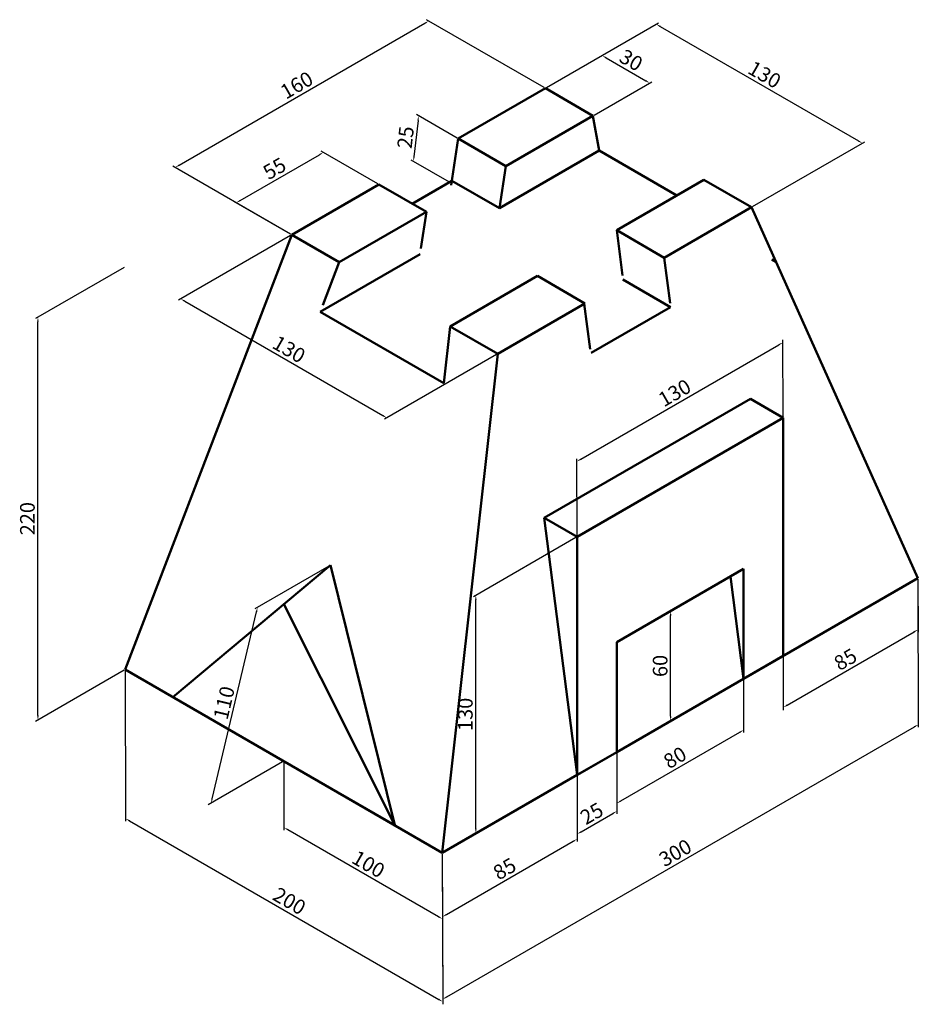
# Model space of a CAD drawing. Units: millimetres. Extents: x 46 to 537, y -102 to 436.
import ezdxf

# ---------------------------------------------------------------- set-up
doc = ezdxf.new("R2010")
doc.units = ezdxf.units.MM
doc.layers.add('M-DIMS', color=3, linetype='Continuous', lineweight=25)
doc.layers.add('M-OUTL', color=7, linetype='Continuous', lineweight=50)
doc.styles.get("Standard").update_dxf_attribs({"font": 'arial.ttf'})
doc.dimstyles.new('ISO-25', dxfattribs={"dimtxt": 8, "dimasz": 2.5, "dimexe": 1.25, "dimexo": 0.625, "dimtad": 1, "dimtxsty": 'Standard', "dimcen": 2.5, "dimadec": 0, "dimazin": 0, "dimtfac": 1, "dimtmove": 0, "dimatfit": 3, "dimfxl": 1, "dimarcsym": 0})

# ---------------------------------------------------------------- blocks, each defined once
blk = doc.blocks.new('*D1')
at = {"layer": 'Defpoints', "color": 0, "transparency": 16777216}
for p in [(333.35, 398.34), (390.34, 401.24), (359.33, 383.34)]:
    blk.add_point(p, dxfattribs=at)
at = {"layer": 'M-DIMS', "color": 0, "lineweight": -2, "transparency": 16777216}
for p, q in [((333.98, 398.7), (365.61, 416.96)), ((366.52, 414.99), (388.17, 402.49)), ((359.96, 383.7), (391.59, 401.96))]:
    blk.add_line(p, q, dxfattribs=at)
at = {"layer": 'M-DIMS', "color": 0, "transparency": 16777216}
for points in [[(366.73, 415.35), (366.32, 414.63), (364.36, 416.24)], [(388.38, 402.85), (387.97, 402.13), (390.34, 401.24)]]:
    blk.add_solid(points, dxfattribs=at)
at = {"layer": 'M-DIMS', "color": 0, "transparency": 16777216, "insert": (379.71, 412.82), "char_height": 8, "attachment_point": 5, "rotation": 330}
blk.add_mtext('30', dxfattribs=at)
blk = doc.blocks.new('*D2')
at = {"layer": 'Defpoints', "color": 0, "transparency": 16777216}
for p in [(333.35, 398.34), (506.56, 368.34), (445.93, 333.34)]:
    blk.add_point(p, dxfattribs=at)
at = {"layer": 'M-DIMS', "color": 0, "lineweight": -2, "transparency": 16777216}
for p, q in [((333.98, 398.7), (395.22, 434.06)), ((396.14, 432.09), (504.39, 369.59)), ((446.56, 333.7), (507.81, 369.06))]:
    blk.add_line(p, q, dxfattribs=at)
at = {"layer": 'M-DIMS', "color": 0, "transparency": 16777216}
for points in [[(396.35, 432.45), (395.93, 431.72), (393.97, 433.34)], [(504.6, 369.95), (504.18, 369.22), (506.56, 368.34)]]:
    blk.add_solid(points, dxfattribs=at)
at = {"layer": 'M-DIMS', "color": 0, "transparency": 16777216, "insert": (452.62, 404.92), "char_height": 8, "attachment_point": 5, "rotation": 330}
blk.add_mtext('130', dxfattribs=at)
blk = doc.blocks.new('*D3')
at = {"layer": 'Defpoints', "color": 0, "transparency": 16777216}
for p in [(212.11, 363.34), (242.42, 345.84), (194.79, 318.34)]:
    blk.add_point(p, dxfattribs=at)
at = {"layer": 'M-DIMS', "color": 0, "lineweight": -2, "transparency": 16777216}
for p, q in [((166.64, 337.09), (209.94, 362.09)), ((241.79, 346.2), (210.86, 364.06)), ((194.16, 318.7), (163.23, 336.56))]:
    blk.add_line(p, q, dxfattribs=at)
at = {"layer": 'M-DIMS', "color": 0, "transparency": 16777216}
for points in [[(209.73, 362.45), (210.15, 361.72), (212.11, 363.34)], [(166.43, 337.45), (166.85, 336.72), (164.48, 335.84)]]:
    blk.add_solid(points, dxfattribs=at)
at = {"layer": 'M-DIMS', "color": 0, "transparency": 16777216, "insert": (185.94, 353.65), "char_height": 8, "attachment_point": 5, "rotation": 30}
blk.add_mtext('55', dxfattribs=at)
blk = doc.blocks.new('*D4')
at = {"layer": 'Defpoints', "color": 0, "transparency": 16777216}
for p in [(285.72, 370.84), (261.3, 358.47), (282.91, 345.99)]:
    blk.add_point(p, dxfattribs=at)
at = {"layer": 'M-DIMS', "color": 0, "lineweight": -2, "transparency": 16777216}
for p, q in [((285.13, 371.18), (262.92, 384)), ((263.82, 380.83), (261.58, 360.96)), ((282.32, 346.33), (260.12, 359.15))]:
    blk.add_line(p, q, dxfattribs=at)
at = {"layer": 'M-DIMS', "color": 0, "transparency": 16777216}
for points in [[(263.41, 380.88), (264.24, 380.78), (264.1, 383.31)], [(261.17, 361), (261.99, 360.91), (261.3, 358.47)]]:
    blk.add_solid(points, dxfattribs=at)
at = {"layer": 'M-DIMS', "color": 0, "transparency": 16777216, "insert": (258.02, 371.42), "char_height": 8, "attachment_point": 5, "rotation": 83.5591}
blk.add_mtext('25', dxfattribs=at)
blk = doc.blocks.new('*D5')
at = {"layer": 'Defpoints', "color": 0, "transparency": 16777216}
for p in [(103.85, 300.84), (56.16, 273.3), (103.85, 80.84)]:
    blk.add_point(p, dxfattribs=at)
at = {"layer": 'M-DIMS', "color": 0, "lineweight": -2, "transparency": 16777216}
for p, q in [((103.23, 300.47), (54.91, 272.58)), ((56.16, 55.8), (56.16, 270.8)), ((103.23, 80.47), (54.91, 52.58))]:
    blk.add_line(p, q, dxfattribs=at)
at = {"layer": 'M-DIMS', "color": 0, "transparency": 16777216}
for points in [[(55.74, 270.8), (56.57, 270.8), (56.16, 273.3)], [(55.74, 55.8), (56.57, 55.8), (56.16, 53.3)]]:
    blk.add_solid(points, dxfattribs=at)
at = {"layer": 'M-DIMS', "color": 0, "transparency": 16777216, "insert": (51.45, 163.3), "char_height": 8, "attachment_point": 5, "rotation": 90}
blk.add_mtext('220', dxfattribs=at)
blk = doc.blocks.new('*D6')
at = {"layer": 'Defpoints', "color": 0, "transparency": 16777216}
for p in [(103.85, 80.84), (277.06, -19.16), (277.29, -100.49)]:
    blk.add_point(p, dxfattribs=at)
at = {"layer": 'M-DIMS', "color": 0, "lineweight": -2, "transparency": 16777216}
for p, q in [((103.86, 80.11), (104.09, -1.93)), ((106.25, -1.74), (275.13, -99.24)), ((277.06, -19.89), (277.3, -101.93))]:
    blk.add_line(p, q, dxfattribs=at)
at = {"layer": 'M-DIMS', "color": 0, "transparency": 16777216}
for points in [[(106.46, -1.38), (106.04, -2.1), (104.09, -0.49)], [(275.33, -98.88), (274.92, -99.6), (277.29, -100.49)]]:
    blk.add_solid(points, dxfattribs=at)
at = {"layer": 'M-DIMS', "color": 0, "transparency": 16777216, "insert": (193.04, -46.41), "char_height": 8, "attachment_point": 5, "rotation": 330}
blk.add_mtext('200', dxfattribs=at)
blk = doc.blocks.new('*D7')
at = {"layer": 'Defpoints', "color": 0, "transparency": 16777216}
for p in [(190.46, 30.84), (190.56, -5.35), (277.06, -19.16)]:
    blk.add_point(p, dxfattribs=at)
at = {"layer": 'M-DIMS', "color": 0, "lineweight": -2, "transparency": 16777216}
for p, q in [((190.46, 30.11), (190.56, -6.8)), ((275, -54.1), (192.72, -6.6)), ((277.06, -19.89), (277.17, -56.8))]:
    blk.add_line(p, q, dxfattribs=at)
at = {"layer": 'M-DIMS', "color": 0, "transparency": 16777216}
for points in [[(192.93, -6.24), (192.52, -6.96), (190.56, -5.35)], [(275.21, -53.74), (274.79, -54.46), (277.16, -55.35)]]:
    blk.add_solid(points, dxfattribs=at)
at = {"layer": 'M-DIMS', "color": 0, "transparency": 16777216, "insert": (236.22, -26.27), "char_height": 8, "attachment_point": 5, "rotation": 330}
blk.add_mtext('100', dxfattribs=at)
blk = doc.blocks.new('*D8')
at = {"layer": 'Defpoints', "color": 0, "transparency": 16777216}
for p in [(215.9, 137.85), (176.17, 114.91), (190.46, 30.84)]:
    blk.add_point(p, dxfattribs=at)
at = {"layer": 'M-DIMS', "color": 0, "lineweight": -2, "transparency": 16777216}
for p, q in [((215.15, 137.42), (174.68, 114.05)), ((151.3, 10.33), (175.59, 112.48)), ((189.71, 30.41), (149.24, 7.04))]:
    blk.add_line(p, q, dxfattribs=at)
at = {"layer": 'M-DIMS', "color": 0, "transparency": 16777216}
for points in [[(175.18, 112.58), (175.99, 112.39), (176.17, 114.91)], [(150.9, 10.43), (151.71, 10.23), (150.73, 7.9)]]:
    blk.add_solid(points, dxfattribs=at)
at = {"layer": 'M-DIMS', "color": 0, "transparency": 16777216, "insert": (158.87, 62.49), "char_height": 8, "attachment_point": 5, "rotation": 76.6272}
blk.add_mtext('110', dxfattribs=at)
blk = doc.blocks.new('*D9')
at = {"layer": 'Defpoints', "color": 0, "transparency": 16777216}
for p in [(350.67, 23.34), (350.77, -11.66), (277.06, -19.16)]:
    blk.add_point(p, dxfattribs=at)
at = {"layer": 'M-DIMS', "color": 0, "lineweight": -2, "transparency": 16777216}
for p, q in [((350.67, 22.61), (350.78, -13.1)), ((279.32, -52.91), (348.61, -12.91)), ((277.06, -19.89), (277.16, -55.6))]:
    blk.add_line(p, q, dxfattribs=at)
at = {"layer": 'M-DIMS', "color": 0, "transparency": 16777216}
for points in [[(348.4, -12.55), (348.81, -13.27), (350.77, -11.66)], [(279.12, -52.55), (279.53, -53.27), (277.16, -54.16)]]:
    blk.add_solid(points, dxfattribs=at)
at = {"layer": 'M-DIMS', "color": 0, "transparency": 16777216, "insert": (311.61, -28.83), "char_height": 8, "attachment_point": 5, "rotation": 30}
blk.add_mtext('85', dxfattribs=at)
blk = doc.blocks.new('*D10')
at = {"layer": 'Defpoints', "color": 0, "transparency": 16777216}
for p in [(441.6, 75.84), (441.68, 47.87), (372.32, 35.84)]:
    blk.add_point(p, dxfattribs=at)
at = {"layer": 'M-DIMS', "color": 0, "lineweight": -2, "transparency": 16777216}
for p, q in [((441.61, 75.11), (441.69, 46.43)), ((374.57, 9.12), (439.52, 46.62)), ((372.32, 35.11), (372.41, 6.43))]:
    blk.add_line(p, q, dxfattribs=at)
at = {"layer": 'M-DIMS', "color": 0, "transparency": 16777216}
for points in [[(439.31, 46.98), (439.73, 46.26), (441.68, 47.87)], [(374.36, 9.48), (374.78, 8.76), (372.4, 7.87)]]:
    blk.add_solid(points, dxfattribs=at)
at = {"layer": 'M-DIMS', "color": 0, "transparency": 16777216, "insert": (404.69, 31.95), "char_height": 8, "attachment_point": 5, "rotation": 30}
blk.add_mtext('80', dxfattribs=at)
blk = doc.blocks.new('*D11')
at = {"layer": 'Defpoints', "color": 0, "transparency": 16777216}
for p in [(536.87, 130.84), (536.95, 102.72), (463.25, 88.34)]:
    blk.add_point(p, dxfattribs=at)
at = {"layer": 'M-DIMS', "color": 0, "lineweight": -2, "transparency": 16777216}
for p, q in [((536.87, 130.11), (536.95, 101.28)), ((465.5, 61.47), (534.78, 101.47)), ((463.26, 87.61), (463.34, 58.78))]:
    blk.add_line(p, q, dxfattribs=at)
at = {"layer": 'M-DIMS', "color": 0, "transparency": 16777216}
for points in [[(534.57, 101.83), (534.99, 101.11), (536.95, 102.72)], [(465.29, 61.83), (465.71, 61.11), (463.33, 60.22)]]:
    blk.add_solid(points, dxfattribs=at)
at = {"layer": 'M-DIMS', "color": 0, "transparency": 16777216, "insert": (497.79, 85.55), "char_height": 8, "attachment_point": 5, "rotation": 30}
blk.add_mtext('85', dxfattribs=at)
blk = doc.blocks.new('*D12')
at = {"layer": 'Defpoints', "color": 0, "transparency": 16777216}
for p in [(372.32, 35.84), (350.67, 23.34), (372.41, 3.54)]:
    blk.add_point(p, dxfattribs=at)
at = {"layer": 'M-DIMS', "color": 0, "lineweight": -2, "transparency": 16777216}
for p, q in [((372.32, 35.11), (372.42, 2.1)), ((350.67, 22.61), (350.77, -10.4)), ((352.93, -7.71), (370.25, 2.29))]:
    blk.add_line(p, q, dxfattribs=at)
at = {"layer": 'M-DIMS', "color": 0, "transparency": 16777216}
for points in [[(370.04, 2.65), (370.46, 1.93), (372.41, 3.54)], [(352.72, -7.35), (353.14, -8.07), (350.76, -8.96)]]:
    blk.add_solid(points, dxfattribs=at)
at = {"layer": 'M-DIMS', "color": 0, "transparency": 16777216, "insert": (359.23, 1.37), "char_height": 8, "attachment_point": 5, "rotation": 30}
blk.add_mtext('25', dxfattribs=at)
blk = doc.blocks.new('*D13')
at = {"layer": 'Defpoints', "color": 0, "transparency": 16777216}
for p in [(536.87, 130.84), (537.1, 50.85), (277.06, -19.16)]:
    blk.add_point(p, dxfattribs=at)
at = {"layer": 'M-DIMS', "color": 0, "lineweight": -2, "transparency": 16777216}
for p, q in [((536.87, 130.11), (537.1, 49.41)), ((279.45, -97.9), (534.93, 49.6)), ((277.06, -19.89), (277.29, -100.59))]:
    blk.add_line(p, q, dxfattribs=at)
at = {"layer": 'M-DIMS', "color": 0, "transparency": 16777216}
for points in [[(534.72, 49.96), (535.14, 49.24), (537.1, 50.85)], [(279.24, -97.54), (279.66, -98.26), (277.29, -99.15)]]:
    blk.add_solid(points, dxfattribs=at)
at = {"layer": 'M-DIMS', "color": 0, "transparency": 16777216, "insert": (404.84, -20.07), "char_height": 8, "attachment_point": 5, "rotation": 30}
blk.add_mtext('300', dxfattribs=at)
blk = doc.blocks.new('*D14')
at = {"layer": 'Defpoints', "color": 0, "transparency": 16777216}
for p in [(350.67, 153.34), (295.39, 121.42), (350.67, 23.34)]:
    blk.add_point(p, dxfattribs=at)
at = {"layer": 'M-DIMS', "color": 0, "lineweight": -2, "transparency": 16777216}
for p, q in [((350.05, 152.97), (294.14, 120.69)), ((295.39, -6.08), (295.39, 118.92)), ((350.05, 22.97), (294.14, -9.31))]:
    blk.add_line(p, q, dxfattribs=at)
at = {"layer": 'M-DIMS', "color": 0, "transparency": 16777216}
for points in [[(294.97, 118.92), (295.8, 118.92), (295.39, 121.42)], [(294.97, -6.08), (295.8, -6.08), (295.39, -8.58)]]:
    blk.add_solid(points, dxfattribs=at)
at = {"layer": 'M-DIMS', "color": 0, "transparency": 16777216, "insert": (290.67, 56.42), "char_height": 8, "attachment_point": 5, "rotation": 90}
blk.add_mtext('130', dxfattribs=at)
blk = doc.blocks.new('*D15')
at = {"layer": 'Defpoints', "color": 0, "transparency": 16777216}
for p in [(463.14, 259.54), (463.25, 218.34), (350.67, 153.34)]:
    blk.add_point(p, dxfattribs=at)
at = {"layer": 'M-DIMS', "color": 0, "lineweight": -2, "transparency": 16777216}
for p, q in [((352.72, 195.79), (460.97, 258.29)), ((463.25, 219.06), (463.13, 260.98)), ((350.67, 154.06), (350.55, 195.98))]:
    blk.add_line(p, q, dxfattribs=at)
at = {"layer": 'M-DIMS', "color": 0, "transparency": 16777216}
for points in [[(460.76, 258.65), (461.18, 257.93), (463.14, 259.54)], [(352.51, 196.15), (352.93, 195.43), (350.55, 194.54)]]:
    blk.add_solid(points, dxfattribs=at)
at = {"layer": 'M-DIMS', "color": 0, "transparency": 16777216, "insert": (404.49, 231.12), "char_height": 8, "attachment_point": 5, "rotation": 30}
blk.add_mtext('130', dxfattribs=at)
blk = doc.blocks.new('*D16')
at = {"layer": 'Defpoints', "color": 0, "transparency": 16777216}
for p in [(269.69, 435.09), (333.35, 398.34), (194.79, 318.34)]:
    blk.add_point(p, dxfattribs=at)
at = {"layer": 'M-DIMS', "color": 0, "lineweight": -2, "transparency": 16777216}
for p, q in [((332.73, 398.7), (268.44, 435.81)), ((133.29, 356.34), (267.52, 433.84)), ((194.16, 318.7), (129.88, 355.81))]:
    blk.add_line(p, q, dxfattribs=at)
at = {"layer": 'M-DIMS', "color": 0, "transparency": 16777216}
for points in [[(267.32, 434.2), (267.73, 433.48), (269.69, 435.09)], [(133.08, 356.7), (133.5, 355.98), (131.13, 355.09)]]:
    blk.add_solid(points, dxfattribs=at)
at = {"layer": 'M-DIMS', "color": 0, "transparency": 16777216, "insert": (198.05, 399.17), "char_height": 8, "attachment_point": 5, "rotation": 30}
blk.add_mtext('160', dxfattribs=at)
blk = doc.blocks.new('*D17')
at = {"layer": 'Defpoints', "color": 0, "transparency": 16777216}
for p in [(194.79, 318.34), (307.37, 253.34), (246.75, 218.34)]:
    blk.add_point(p, dxfattribs=at)
at = {"layer": 'M-DIMS', "color": 0, "lineweight": -2, "transparency": 16777216}
for p, q in [((194.16, 317.97), (132.91, 282.61)), ((136.33, 282.09), (244.58, 219.59)), ((306.74, 252.97), (245.5, 217.61))]:
    blk.add_line(p, q, dxfattribs=at)
at = {"layer": 'M-DIMS', "color": 0, "transparency": 16777216}
for points in [[(136.54, 282.45), (136.12, 281.72), (134.16, 283.34)], [(244.79, 219.95), (244.37, 219.22), (246.75, 218.34)]]:
    blk.add_solid(points, dxfattribs=at)
at = {"layer": 'M-DIMS', "color": 0, "transparency": 16777216, "insert": (192.81, 254.92), "char_height": 8, "attachment_point": 5, "rotation": 330}
blk.add_mtext('130', dxfattribs=at)
blk = doc.blocks.new('*D18')
at = {"layer": 'Defpoints', "color": 0, "transparency": 16777216}
for p in [(401.81, 112.86), (372.32, 95.84), (372.32, 35.84)]:
    blk.add_point(p, dxfattribs=at)
at = {"layer": 'M-DIMS', "color": 0, "lineweight": -2, "transparency": 16777216}
for p, q in [((372.95, 96.2), (403.06, 113.58)), ((401.81, 55.36), (401.81, 110.36)), ((372.95, 36.2), (403.06, 53.58))]:
    blk.add_line(p, q, dxfattribs=at)
at = {"layer": 'M-DIMS', "color": 0, "transparency": 16777216}
for points in [[(401.4, 110.36), (402.23, 110.36), (401.81, 112.86)], [(401.4, 55.36), (402.23, 55.36), (401.81, 52.86)]]:
    blk.add_solid(points, dxfattribs=at)
at = {"layer": 'M-DIMS', "color": 0, "transparency": 16777216, "insert": (397.1, 82.86), "char_height": 8, "attachment_point": 5, "rotation": 90}
blk.add_mtext('60', dxfattribs=at)

msp = doc.modelspace()

# ---------------------------------------------------------------- linework, layer by layer
at = {"layer": 'M-OUTL'}
for p, q in [((285.719, 370.835), (333.351, 398.335)), ((333.351, 398.335), (359.331, 383.335)), ((359.331, 383.335), (311.7, 355.835)), ((359.331, 383.335), (362.776, 364.301)), ((281.914, 345.415), (285.719, 370.835)), ((311.7, 355.835), (285.719, 370.835)), ((308.256, 332.824), (362.776, 364.301)), ((362.776, 364.301), (405.191, 339.812)), ((311.7, 355.835), (308.256, 332.824)), ((194.787, 318.335), (242.418, 345.835)), ((194.787, 318.335), (242.418, 345.835)), ((242.418, 345.835), (268.399, 330.835)), ((260.624, 335.324), (282.275, 347.824)), ((308.256, 332.824), (282.275, 347.824)), ((372.322, 320.835), (419.953, 348.335)), ((419.953, 348.335), (445.934, 333.335)), ((268.399, 330.835), (220.767, 303.335)), ((265.419, 310.928), (268.399, 330.835)), ((445.934, 333.335), (398.303, 305.835)), ((445.934, 333.335), (536.867, 130.835)), ((194.787, 318.335), (103.854, 80.835)), ((220.767, 303.335), (194.787, 318.335)), ((398.303, 305.835), (372.322, 320.835)), ((375.489, 296.02), (372.322, 320.835)), ((210.434, 276.346), (264.954, 307.824)), ((220.767, 303.335), (211.828, 279.988)), ((401.47, 281.02), (398.303, 305.835)), ((457.166, 304.82), (459.289, 303.594)), ((329.021, 295.835), (281.389, 268.335)), ((355.001, 280.835), (329.021, 295.835)), ((401.747, 278.846), (375.766, 293.846)), ((307.37, 253.335), (355.001, 280.835)), ((354.65, 280.632), (354.568, 281.085)), ((357.854, 255.838), (354.65, 280.632)), ((354.65, 280.632), (357.854, 255.838)), ((277.945, 237.369), (210.434, 276.346)), ((401.747, 278.846), (358.446, 253.846)), ((281.389, 268.335), (277.945, 237.369)), ((281.389, 268.335), (307.37, 253.335)), ((307.37, 253.335), (277.059, -19.165)), ((332.76, 163.676), (445.344, 228.676)), ((445.344, 228.676), (463.255, 218.335)), ((350.671, 153.335), (463.255, 218.335)), ((463.255, 218.335), (463.255, 88.335)), ((390.746, 176.472), (390.716, 176.707)), ((390.716, 176.707), (390.934, 176.581)), ((350.671, 23.335), (332.76, 163.676)), ((350.671, 153.335), (332.76, 163.676)), ((350.671, 23.335), (350.671, 153.335)), ((129.835, 65.835), (215.898, 137.853)), ((215.898, 137.853), (251.078, -4.165)), ((372.322, 95.835), (441.604, 135.835)), ((441.604, 75.835), (441.604, 135.835)), ((441.604, 75.835), (434.472, 131.717)), ((536.867, 130.835), (441.604, 75.835)), ((463.255, 88.335), (536.867, 130.835)), ((190.457, 116.563), (251.078, -4.165)), ((372.322, 35.835), (372.322, 95.835)), ((463.255, 88.335), (441.604, 75.835)), ((103.854, 80.835), (277.059, -19.165)), ((372.322, 35.835), (441.604, 75.835)), ((251.078, -4.165), (129.835, 65.835)), ((277.059, -19.165), (372.322, 35.835)), ((350.671, 23.335), (372.322, 35.835)), ((350.671, 23.335), (277.059, -19.165))]:
    msp.add_line(p, q, dxfattribs=at)

# ---------------------------------------------------------------- dimensions: what is measured, and where the dimension line sits
at = {"layer": 'M-DIMS'}
for p1, p2, distance, picture, middle in [((194.787, 318.335), (333.351, 398.335), 63.661, '*D16', (198.053, 399.168)), ((333.351, 398.335), (445.934, 333.335), 60.622, '*D2', (452.62, 404.916)), ((333.351, 398.335), (359.331, 383.335), 31.008, '*D1', (379.705, 412.819)), ((285.719, 370.835), (282.915, 345.993), -22.878, '*D4', (258.023, 371.421)), ((194.787, 318.335), (242.418, 345.835), 30.311, '*D3', (185.945, 353.65)), ((194.787, 318.335), (307.37, 253.335), -60.622, '*D17', (192.813, 254.916)), ((103.854, 80.835), (103.854, 300.835), 47.697, '*D5', (51.447, 163.297)), ((350.671, 153.335), (463.255, 218.335), 35.745, '*D15', (404.489, 231.123)), ((350.671, 23.335), (350.671, 153.335), 55.285, '*D14', (290.674, 56.416)), ((190.457, 30.835), (215.898, 137.853), 33.348, '*D8', (158.865, 62.495)), ((277.059, -19.165), (536.867, 130.835), -69.381, '*D13', (404.835, -20.066)), ((463.255, 88.335), (536.867, 130.835), -24.389, '*D11', (497.786, 85.548)), ((372.322, 35.835), (372.322, 95.835), -29.492, '*D18', (397.104, 82.862)), ((103.854, 80.835), (277.059, -19.165), -70.31, '*D6', (193.044, -46.408)), ((372.322, 35.835), (441.604, 75.835), -24.261, '*D10', (404.688, 31.945)), ((350.671, 23.335), (372.322, 35.835), -28.011, '*D12', (359.234, 1.372)), ((277.059, -19.165), (190.457, 30.835), 31.288, '*D7', (236.216, -26.275)), ((277.059, -19.165), (350.671, 23.335), -30.359, '*D9', (311.61, -28.834))]:
    dim = msp.add_aligned_dim(p1=p1, p2=p2, distance=distance, dimstyle='ISO-25', override={"dimclrd": 0, "dimclre": 0, "dimclrt": 0}, dxfattribs=at)
    dim.commit()
    dim.dimension.update_dxf_attribs({"geometry": picture, "text_midpoint": middle})

doc.saveas('drawing.dxf')
